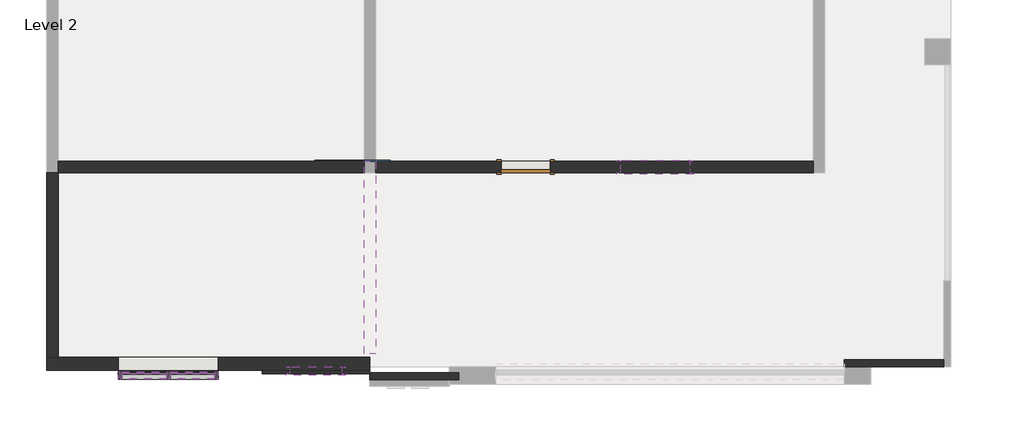
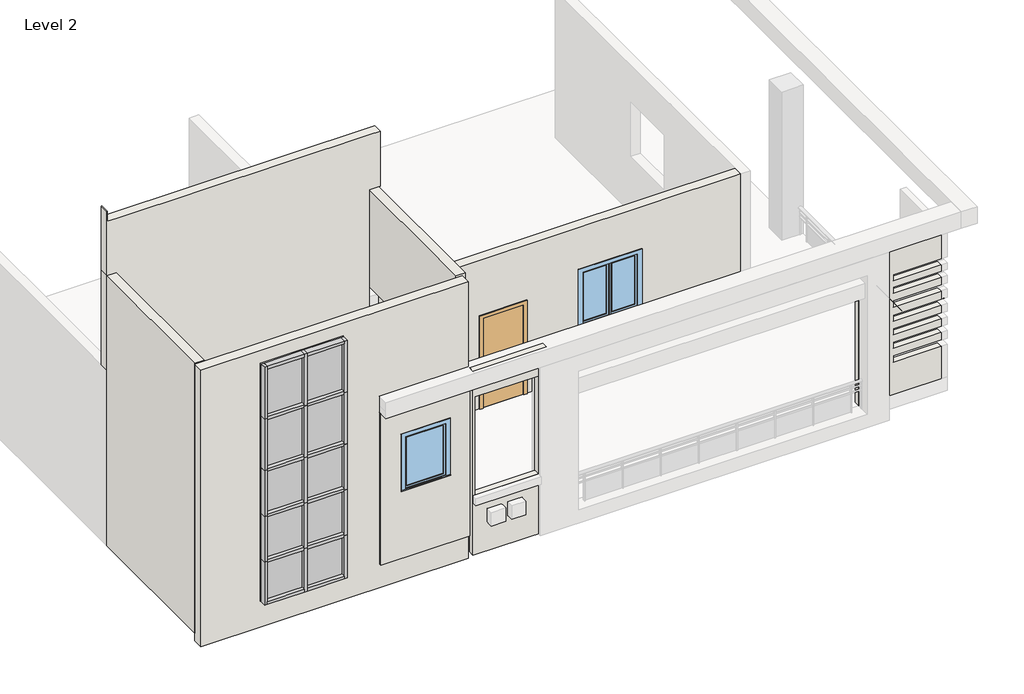
# One storey, part 1 of 2: 27 members, 10 plates, 8 walls, 3 windows, 1 door.
"""IFC4 building model written with IfcOpenShell, lengths in millimetres."""

from ifc_helpers import new_model, si_unit, frame, origin, place, context, project, spatial, polyline, outline, extrude, faceted_brep, transform, mapped, element, save
from components import door_10fd3a06, member_c3a135b3, member_e9460d8e, member_90be0342, member_476d3acb, member_bc9734be, member_9ad71e68, member_76e31e9c, member_801d2a92, system_panel_glazed_0c055d28, system_panel_glazed_6fa9ab24, system_panel_glazed_6a49b045, system_panel_glazed_66480490, window_0862ab64, window_2df9a94c

model = new_model("IFC4")

# Units and contexts
model_context = context("Model", 3, world=origin())
ifc_project = project(units=[si_unit("LENGTHUNIT", "METRE", prefix="MILLI")], contexts=[model_context])

# Site, building, storey
site = spatial("IfcSite", under=ifc_project)
building = spatial("IfcBuilding", under=site)
storey = spatial("IfcBuildingStorey", under=building, Name="Level 2", Elevation=3657.6)

# Door
placement = place(None, origin())
door_shape = door_10fd3a06(model_context)
element("IfcDoor", 1, ObjectType="Door-Single-Panel : 34\" x 80\"", at=placement, inside=storey, context=model_context, shape_type="MappedRepresentation", body=[
    mapped(door_shape, transform((-5364.932483, -170.4259649, 3962.4), x_axis=(-1.0, 0.0, 0.0), y_axis=(0.0, -1.0, 0.0), z_axis=(0.0, 0.0, 1.0))),
])

# Members
member_shape = member_c3a135b3(model_context)
element("IfcMember", 2, ObjectType="Rectangular Mullion : 2.5\" x 5\" rectangular", at=placement, inside=storey, context=model_context, shape_type="MappedRepresentation", body=[
    mapped(member_shape, transform((-11644.6696597, -3853.4259649, 4077.497679), x_axis=(0.0, 0.0, -1.0), y_axis=(0.0, -1.0, 0.0), z_axis=(-1.0, 0.0, 0.0))),
])
element("IfcMember", 3, ObjectType="Rectangular Mullion : 2.5\" x 5\" rectangular", at=placement, inside=storey, context=model_context, shape_type="MappedRepresentation", body=[
    mapped(member_shape, transform((-12496.8288845, -3853.4259649, 4077.497679), x_axis=(0.0, 0.0, -1.0), y_axis=(0.0, -1.0, 0.0), z_axis=(-1.0, 0.0, 0.0))),
])
element("IfcMember", 4, ObjectType="Rectangular Mullion : 2.5\" x 5\" rectangular", at=placement, inside=storey, context=model_context, shape_type="MappedRepresentation", body=[
    mapped(member_shape, transform((-11708.1696597, -3853.4259649, 9448.8), x_axis=(0.0, 0.0, 1.0), y_axis=(0.0, -1.0, 0.0), z_axis=(1.0, 0.0, 0.0))),
])
element("IfcMember", 5, ObjectType="Rectangular Mullion : 2.5\" x 5\" rectangular", at=placement, inside=storey, context=model_context, shape_type="MappedRepresentation", body=[
    mapped(member_shape, transform((-10856.0104349, -3853.4259649, 9448.8), x_axis=(0.0, 0.0, 1.0), y_axis=(0.0, -1.0, 0.0), z_axis=(1.0, 0.0, 0.0))),
])
member_2_shape = member_e9460d8e(model_context)
element("IfcMember", 6, ObjectType="Rectangular Mullion : 2.5\" x 5\" rectangular", at=placement, inside=storey, context=model_context, shape_type="MappedRepresentation", body=[
    mapped(member_2_shape, transform((-11676.4196597, -3853.4259649, 8280.4), x_axis=(1.0, 0.0, 0.0), y_axis=(0.0, -1.0, 0.0), z_axis=(0.0, 0.0, -1.0))),
])
member_3_shape = member_90be0342(model_context)
element("IfcMember", 7, ObjectType="Rectangular Mullion : 2.5\" x 5\" rectangular", at=placement, inside=storey, context=model_context, shape_type="MappedRepresentation", body=[
    mapped(member_3_shape, transform((-10856.0104349, -3853.4259649, 8280.4), x_axis=(0.0, 0.0, 1.0), y_axis=(0.0, -1.0, 0.0), z_axis=(1.0, 0.0, 0.0))),
])
element("IfcMember", 8, ObjectType="Rectangular Mullion : 2.5\" x 5\" rectangular", at=placement, inside=storey, context=model_context, shape_type="MappedRepresentation", body=[
    mapped(member_3_shape, transform((-11708.1696597, -3853.4259649, 8280.4), x_axis=(0.0, 0.0, 1.0), y_axis=(0.0, -1.0, 0.0), z_axis=(1.0, 0.0, 0.0))),
])
element("IfcMember", 9, ObjectType="Rectangular Mullion : 2.5\" x 5\" rectangular", at=placement, inside=storey, context=model_context, shape_type="MappedRepresentation", body=[
    mapped(member_3_shape, transform((-10856.0104349, -3853.4259649, 7112.0), x_axis=(0.0, 0.0, 1.0), y_axis=(0.0, -1.0, 0.0), z_axis=(1.0, 0.0, 0.0))),
])
element("IfcMember", 10, ObjectType="Rectangular Mullion : 2.5\" x 5\" rectangular", at=placement, inside=storey, context=model_context, shape_type="MappedRepresentation", body=[
    mapped(member_3_shape, transform((-11708.1696597, -3853.4259649, 7112.0), x_axis=(0.0, 0.0, 1.0), y_axis=(0.0, -1.0, 0.0), z_axis=(1.0, 0.0, 0.0))),
])
element("IfcMember", 11, ObjectType="Rectangular Mullion : 2.5\" x 5\" rectangular", at=placement, inside=storey, context=model_context, shape_type="MappedRepresentation", body=[
    mapped(member_3_shape, transform((-10856.0104349, -3853.4259649, 6083.565893), x_axis=(0.0, 0.0, 1.0), y_axis=(0.0, -1.0, 0.0), z_axis=(1.0, 0.0, 0.0))),
])
element("IfcMember", 12, ObjectType="Rectangular Mullion : 2.5\" x 5\" rectangular", at=placement, inside=storey, context=model_context, shape_type="MappedRepresentation", body=[
    mapped(member_3_shape, transform((-11708.1696597, -3853.4259649, 6083.565893), x_axis=(0.0, 0.0, 1.0), y_axis=(0.0, -1.0, 0.0), z_axis=(1.0, 0.0, 0.0))),
])
element("IfcMember", 13, ObjectType="Rectangular Mullion : 2.5\" x 5\" rectangular", at=placement, inside=storey, context=model_context, shape_type="MappedRepresentation", body=[
    mapped(member_3_shape, transform((-10856.0104349, -3853.4259649, 5055.131786), x_axis=(0.0, 0.0, 1.0), y_axis=(0.0, -1.0, 0.0), z_axis=(1.0, 0.0, 0.0))),
])
element("IfcMember", 14, ObjectType="Rectangular Mullion : 2.5\" x 5\" rectangular", at=placement, inside=storey, context=model_context, shape_type="MappedRepresentation", body=[
    mapped(member_3_shape, transform((-11708.1696597, -3853.4259649, 5055.131786), x_axis=(0.0, 0.0, 1.0), y_axis=(0.0, -1.0, 0.0), z_axis=(1.0, 0.0, 0.0))),
])
member_4_shape = member_476d3acb(model_context)
element("IfcMember", 15, ObjectType="Rectangular Mullion : 2.5\" x 5\" rectangular", at=placement, inside=storey, context=model_context, shape_type="MappedRepresentation", body=[
    mapped(member_4_shape, transform((-12560.3288845, -3853.4259649, 9448.8), x_axis=(-1.0, 0.0, 0.0), y_axis=(0.0, -1.0, 0.0), z_axis=(0.0, 0.0, 1.0))),
])
element("IfcMember", 16, ObjectType="Rectangular Mullion : 2.5\" x 5\" rectangular", at=placement, inside=storey, context=model_context, shape_type="MappedRepresentation", body=[
    mapped(member_4_shape, transform((-10792.5104349, -3853.4259649, 8280.4), x_axis=(1.0, 0.0, 0.0), y_axis=(0.0, -1.0, 0.0), z_axis=(0.0, 0.0, -1.0))),
])
element("IfcMember", 17, ObjectType="Rectangular Mullion : 2.5\" x 5\" rectangular", at=placement, inside=storey, context=model_context, shape_type="MappedRepresentation", body=[
    mapped(member_2_shape, transform((-11676.4196597, -3853.4259649, 7112.0), x_axis=(1.0, 0.0, 0.0), y_axis=(0.0, -1.0, 0.0), z_axis=(0.0, 0.0, -1.0))),
])
element("IfcMember", 18, ObjectType="Rectangular Mullion : 2.5\" x 5\" rectangular", at=placement, inside=storey, context=model_context, shape_type="MappedRepresentation", body=[
    mapped(member_4_shape, transform((-12560.3288845, -3853.4259649, 8280.4), x_axis=(-1.0, 0.0, 0.0), y_axis=(0.0, -1.0, 0.0), z_axis=(0.0, 0.0, 1.0))),
])
element("IfcMember", 19, ObjectType="Rectangular Mullion : 2.5\" x 5\" rectangular", at=placement, inside=storey, context=model_context, shape_type="MappedRepresentation", body=[
    mapped(member_4_shape, transform((-10792.5104349, -3853.4259649, 7112.0), x_axis=(1.0, 0.0, 0.0), y_axis=(0.0, -1.0, 0.0), z_axis=(0.0, 0.0, -1.0))),
])
member_5_shape = member_bc9734be(model_context)
element("IfcMember", 20, ObjectType="Rectangular Mullion : 2.5\" x 5\" rectangular", at=placement, inside=storey, context=model_context, shape_type="MappedRepresentation", body=[
    mapped(member_5_shape, transform((-11676.4196597, -3853.4259649, 6083.565893), x_axis=(1.0, 0.0, 0.0), y_axis=(0.0, -1.0, 0.0), z_axis=(0.0, 0.0, -1.0))),
])
element("IfcMember", 21, ObjectType="Rectangular Mullion : 2.5\" x 5\" rectangular", at=placement, inside=storey, context=model_context, shape_type="MappedRepresentation", body=[
    mapped(member_5_shape, transform((-11676.4196597, -3853.4259649, 5055.131786), x_axis=(1.0, 0.0, 0.0), y_axis=(0.0, -1.0, 0.0), z_axis=(0.0, 0.0, -1.0))),
])
member_6_shape = member_9ad71e68(model_context)
element("IfcMember", 22, ObjectType="Rectangular Mullion : 2.5\" x 5\" rectangular", at=placement, inside=storey, context=model_context, shape_type="MappedRepresentation", body=[
    mapped(member_6_shape, transform((-12560.3288845, -3853.4259649, 7112.0), x_axis=(-1.0, 0.0, 0.0), y_axis=(0.0, -1.0, 0.0), z_axis=(0.0, 0.0, 1.0))),
])
element("IfcMember", 23, ObjectType="Rectangular Mullion : 2.5\" x 5\" rectangular", at=placement, inside=storey, context=model_context, shape_type="MappedRepresentation", body=[
    mapped(member_6_shape, transform((-12560.3288845, -3853.4259649, 6083.565893), x_axis=(-1.0, 0.0, 0.0), y_axis=(0.0, -1.0, 0.0), z_axis=(0.0, 0.0, 1.0))),
])
element("IfcMember", 24, ObjectType="Rectangular Mullion : 2.5\" x 5\" rectangular", at=placement, inside=storey, context=model_context, shape_type="MappedRepresentation", body=[
    mapped(member_6_shape, transform((-10792.5104349, -3853.4259649, 6083.565893), x_axis=(1.0, 0.0, 0.0), y_axis=(0.0, -1.0, 0.0), z_axis=(0.0, 0.0, -1.0))),
])
element("IfcMember", 25, ObjectType="Rectangular Mullion : 2.5\" x 5\" rectangular", at=placement, inside=storey, context=model_context, shape_type="MappedRepresentation", body=[
    mapped(member_6_shape, transform((-10792.5104349, -3853.4259649, 5055.131786), x_axis=(1.0, 0.0, 0.0), y_axis=(0.0, -1.0, 0.0), z_axis=(0.0, 0.0, -1.0))),
])
member_7_shape = member_76e31e9c(model_context)
element("IfcMember", 26, ObjectType="Rectangular Mullion : 2.5\" x 5\" rectangular", at=placement, inside=storey, context=model_context, shape_type="MappedRepresentation", body=[
    mapped(member_7_shape, transform((-11676.4196597, -3853.4259649, 4077.497679), x_axis=(1.0, 0.0, 0.0), y_axis=(0.0, -1.0, 0.0), z_axis=(0.0, 0.0, -1.0))),
])
member_8_shape = member_801d2a92(model_context)
element("IfcMember", 27, ObjectType="Rectangular Mullion : 2.5\" x 5\" rectangular", at=placement, inside=storey, context=model_context, shape_type="MappedRepresentation", body=[
    mapped(member_8_shape, transform((-10792.5104349, -3853.4259649, 4077.497679), x_axis=(1.0, 0.0, 0.0), y_axis=(0.0, -1.0, 0.0), z_axis=(0.0, 0.0, -1.0))),
])
element("IfcMember", 28, ObjectType="Rectangular Mullion : 2.5\" x 5\" rectangular", at=placement, inside=storey, context=model_context, shape_type="MappedRepresentation", body=[
    mapped(member_8_shape, transform((-12560.3288845, -3853.4259649, 5055.131786), x_axis=(-1.0, 0.0, 0.0), y_axis=(0.0, -1.0, 0.0), z_axis=(0.0, 0.0, 1.0))),
])

# Plates
system_panel_glazed_shape = system_panel_glazed_0c055d28(model_context)
element("IfcPlate", 29, ObjectType="System Panel : Glazed", at=placement, inside=storey, context=model_context, shape_type="MappedRepresentation", body=[
    mapped(system_panel_glazed_shape, transform((-12102.4992721, -3853.4259649, 8312.15), x_axis=(1.0, 0.0, 0.0), y_axis=(0.0, 1.0, 0.0), z_axis=(0.0, 0.0, 1.0))),
])
element("IfcPlate", 30, ObjectType="System Panel : Glazed", at=placement, inside=storey, context=model_context, shape_type="MappedRepresentation", body=[
    mapped(system_panel_glazed_shape, transform((-11250.3400473, -3853.4259649, 8312.15), x_axis=(1.0, 0.0, 0.0), y_axis=(0.0, 1.0, 0.0), z_axis=(0.0, 0.0, 1.0))),
])
system_panel_glazed_2_shape = system_panel_glazed_6fa9ab24(model_context)
element("IfcPlate", 31, ObjectType="System Panel : Glazed", at=placement, inside=storey, context=model_context, shape_type="MappedRepresentation", body=[
    mapped(system_panel_glazed_2_shape, transform((-12102.4992721, -3853.4259649, 7143.75), x_axis=(1.0, 0.0, 0.0), y_axis=(0.0, 1.0, 0.0), z_axis=(0.0, 0.0, 1.0))),
])
element("IfcPlate", 32, ObjectType="System Panel : Glazed", at=placement, inside=storey, context=model_context, shape_type="MappedRepresentation", body=[
    mapped(system_panel_glazed_2_shape, transform((-11250.3400473, -3853.4259649, 7143.75), x_axis=(1.0, 0.0, 0.0), y_axis=(0.0, 1.0, 0.0), z_axis=(0.0, 0.0, 1.0))),
])
system_panel_glazed_3_shape = system_panel_glazed_6a49b045(model_context)
element("IfcPlate", 33, ObjectType="System Panel : Glazed", at=placement, inside=storey, context=model_context, shape_type="MappedRepresentation", body=[
    mapped(system_panel_glazed_3_shape, transform((-12102.4992721, -3853.4259649, 6115.315893), x_axis=(1.0, 0.0, 0.0), y_axis=(0.0, 1.0, 0.0), z_axis=(0.0, 0.0, 1.0))),
])
element("IfcPlate", 34, ObjectType="System Panel : Glazed", at=placement, inside=storey, context=model_context, shape_type="MappedRepresentation", body=[
    mapped(system_panel_glazed_3_shape, transform((-11250.3400473, -3853.4259649, 6115.315893), x_axis=(1.0, 0.0, 0.0), y_axis=(0.0, 1.0, 0.0), z_axis=(0.0, 0.0, 1.0))),
])
element("IfcPlate", 35, ObjectType="System Panel : Glazed", at=placement, inside=storey, context=model_context, shape_type="MappedRepresentation", body=[
    mapped(system_panel_glazed_3_shape, transform((-12102.4992721, -3853.4259649, 5086.881786), x_axis=(1.0, 0.0, 0.0), y_axis=(0.0, 1.0, 0.0), z_axis=(0.0, 0.0, 1.0))),
])
element("IfcPlate", 36, ObjectType="System Panel : Glazed", at=placement, inside=storey, context=model_context, shape_type="MappedRepresentation", body=[
    mapped(system_panel_glazed_3_shape, transform((-11250.3400473, -3853.4259649, 5086.881786), x_axis=(1.0, 0.0, 0.0), y_axis=(0.0, 1.0, 0.0), z_axis=(0.0, 0.0, 1.0))),
])
system_panel_glazed_4_shape = system_panel_glazed_66480490(model_context)
element("IfcPlate", 37, ObjectType="System Panel : Glazed", at=placement, inside=storey, context=model_context, shape_type="MappedRepresentation", body=[
    mapped(system_panel_glazed_4_shape, transform((-12102.4992721, -3853.4259649, 4140.997679), x_axis=(1.0, 0.0, 0.0), y_axis=(0.0, 1.0, 0.0), z_axis=(0.0, 0.0, 1.0))),
])
element("IfcPlate", 38, ObjectType="System Panel : Glazed", at=placement, inside=storey, context=model_context, shape_type="MappedRepresentation", body=[
    mapped(system_panel_glazed_4_shape, transform((-11250.3400473, -3853.4259649, 4140.997679), x_axis=(1.0, 0.0, 0.0), y_axis=(0.0, 1.0, 0.0), z_axis=(0.0, 0.0, 1.0))),
])

# Walls
element("IfcWall", 39, ObjectType="Generic - 4\" Brick", at=placement, inside=storey, context=model_context, shape_type="SweptSolid", body=[
    extrude(outline(polyline([(4035.6432835, -10021.1728698), (4035.6432835, -8116.1728698), (7457.6935311, -8116.1728698), (7457.6935311, -10021.1728698), (4035.6432835, -10021.1728698)]), holes=[polyline([(6780.679659, -9525.8728698), (6780.679659, -8611.4728698), (5561.479659, -8611.4728698), (5561.479659, -9525.8728698), (6780.679659, -9525.8728698)])]), frame((0.0, -3823.1106886, 0.0), z_axis=(0.0, 1.0, 0.0), x_axis=(0.0, 0.0, 1.0)), (0.0, 0.0, 1.0), 101.6),
])
element("IfcWall", 40, ObjectType="Generic - 5\"", at=placement, inside=storey, context=model_context, shape_type="SweptSolid", body=[
    extrude(outline(polyline([(7820.7521516, -8116.1728698), (3657.6, -8116.1728698), (3657.6, -6547.7228698), (7820.7521516, -6547.7228698), (7820.7521516, -8116.1728698)]), holes=[polyline([(7217.8061863, -6719.1728698), (5010.4540348, -6719.1728698), (5010.4540348, -8065.3728698), (7217.8061863, -8065.3728698), (7217.8061863, -6719.1728698)])]), frame((0.0, -3929.6259649, 0.0), z_axis=(0.0, 1.0, 0.0), x_axis=(0.0, 0.0, 1.0)), (0.0, 0.0, 1.0), 127.0),
])
element("IfcWall", 41, ObjectType="Generic - 5\"", at=placement, inside=storey, context=model_context, shape_type="Brep", body=[
    faceted_brep([(258.2694807, -3701.0259649, 3962.4), (2018.4271302, -3701.0259649, 3962.4), (2018.4271302, -3701.0259649, 4691.6184058), (994.8694807, -3701.0259649, 4691.6184058), (994.8694807, -3701.0259649, 4836.3196283), (2018.4271302, -3701.0259649, 4836.3196283), (2018.4271302, -3701.0259649, 5009.1184058), (994.8694807, -3701.0259649, 5009.1184058), (994.8694807, -3701.0259649, 5141.1196283), (2018.4271302, -3701.0259649, 5141.1196283), (2018.4271302, -3701.0259649, 5313.9184058), (994.8694807, -3701.0259649, 5313.9184058), (994.8694807, -3701.0259649, 5445.9196283), (2018.4271302, -3701.0259649, 5445.9196283), (2018.4271302, -3701.0259649, 5618.7184058), (994.8694807, -3701.0259649, 5618.7184058), (994.8694807, -3701.0259649, 5750.7196283), (2081.9271302, -3701.0259649, 5750.7196283), (2081.9271302, -3701.0259649, 5753.1), (2018.4271302, -3701.0259649, 5753.1), (2018.4271302, -3701.0259649, 5936.2184058), (994.8694807, -3701.0259649, 5936.2184058), (994.8694807, -3701.0259649, 6080.9196283), (2018.4271302, -3701.0259649, 6080.9196283), (2018.4271302, -3701.0259649, 6253.7184058), (994.8694807, -3701.0259649, 6253.7184058), (994.8694807, -3701.0259649, 6385.7196283), (2018.4271302, -3701.0259649, 6385.7196283), (2018.4271302, -3701.0259649, 6533.1184058), (994.8694807, -3701.0259649, 6533.1184058), (994.8694807, -3701.0259649, 6665.1196283), (2018.4271302, -3701.0259649, 6665.1196283), (2018.4271302, -3701.0259649, 7315.2), (258.2694807, -3701.0259649, 7315.2), (258.2694807, -3574.0259649, 3962.4), (258.2694807, -3574.0259649, 7315.2), (2018.4271302, -3574.0259649, 7315.2), (2018.4271302, -3574.0259649, 6665.1196283), (994.8694807, -3574.0259649, 6665.1196283), (994.8694807, -3574.0259649, 6533.1184058), (2018.4271302, -3574.0259649, 6533.1184058), (2018.4271302, -3574.0259649, 6385.7196283), (994.8694807, -3574.0259649, 6385.7196283), (994.8694807, -3574.0259649, 6253.7184058), (2018.4271302, -3574.0259649, 6253.7184058), (2018.4271302, -3574.0259649, 6080.9196283), (994.8694807, -3574.0259649, 6080.9196283), (994.8694807, -3574.0259649, 5936.2184058), (2018.4271302, -3574.0259649, 5936.2184058), (2018.4271302, -3574.0259649, 5753.1), (2081.9271302, -3574.0259649, 5753.1), (2081.9271302, -3574.0259649, 5750.7196283), (994.8694807, -3574.0259649, 5750.7196283), (994.8694807, -3574.0259649, 5618.7184058), (2018.4271302, -3574.0259649, 5618.7184058), (2018.4271302, -3574.0259649, 5445.9196283), (994.8694807, -3574.0259649, 5445.9196283), (994.8694807, -3574.0259649, 5313.9184058), (2018.4271302, -3574.0259649, 5313.9184058), (2018.4271302, -3574.0259649, 5141.1196283), (994.8694807, -3574.0259649, 5141.1196283), (994.8694807, -3574.0259649, 5009.1184058), (2018.4271302, -3574.0259649, 5009.1184058), (2018.4271302, -3574.0259649, 4836.3196283), (994.8694807, -3574.0259649, 4836.3196283), (994.8694807, -3574.0259649, 4691.6184058), (2018.4271302, -3574.0259649, 4691.6184058), (2018.4271302, -3574.0259649, 3962.4), (2018.4271302, -3637.5259649, 6080.9196283), (2018.4271302, -3637.5259649, 6385.7196283)], [[[0, 1, 2, 3, 4, 5, 6, 7, 8, 9, 10, 11, 12, 13, 14, 15, 16, 17, 18, 19, 20, 21, 22, 23, 24, 25, 26, 27, 28, 29, 30, 31, 32, 33]], [[34, 35, 36, 37, 38, 39, 40, 41, 42, 43, 44, 45, 46, 47, 48, 49, 50, 51, 52, 53, 54, 55, 56, 57, 58, 59, 60, 61, 62, 63, 64, 65, 66, 67]], [[1, 0, 34, 67]], [[33, 32, 36, 35]], [[0, 33, 35, 34]], [[3, 2, 66, 65]], [[4, 3, 65, 64]], [[5, 4, 64, 63]], [[7, 6, 62, 61]], [[8, 7, 61, 60]], [[9, 8, 60, 59]], [[11, 10, 58, 57]], [[12, 11, 57, 56]], [[13, 12, 56, 55]], [[15, 14, 54, 53]], [[16, 15, 53, 52]], [[17, 16, 52, 51]], [[21, 20, 48, 47]], [[22, 21, 47, 46]], [[23, 22, 46, 45, 68]], [[25, 24, 44, 43]], [[26, 25, 43, 42]], [[27, 26, 42, 41, 69]], [[29, 28, 40, 39]], [[30, 29, 39, 38]], [[31, 30, 38, 37]], [[18, 17, 51, 50]], [[49, 19, 18, 50]], [[2, 1, 67, 66]], [[6, 5, 63, 62]], [[10, 9, 59, 58]], [[14, 13, 55, 54]], [[20, 19, 49, 48]], [[24, 23, 68, 45, 44]], [[28, 27, 69, 41, 40]], [[32, 31, 37, 36]]]),
])
element("IfcWall", 42, ObjectType="Generic - 8\"", at=placement, inside=storey, context=model_context, shape_type="Brep", body=[
    faceted_brep([(-8217.7728698, -68.8259649, 3657.6), (-13621.6228698, -68.8259649, 3657.6), (-13621.6228698, -68.8259649, 7620.0), (-13654.5805193, -68.8259649, 7620.0), (-13806.9805193, -68.8259649, 7620.0), (-13829.2055193, -68.8259649, 7620.0), (-13829.2055193, -68.8259649, 9753.6), (-13824.8228698, -68.8259649, 9753.6), (-13824.8228698, -68.8259649, 11202.4428486), (-13810.1555193, -68.8259649, 11202.4428486), (-13810.1555193, -68.8259649, 10972.8), (-7989.1728698, -68.8259649, 10972.8), (-7989.1728698, -68.8259649, 9731.3133194), (-8014.5728698, -68.8259649, 9731.3133194), (-8217.7728698, -68.8259649, 9731.3133194), (-8217.7728698, -68.8259649, 7542.338929), (-8217.7728698, -68.8259649, 6108.5737543), (-9030.5728698, -68.8259649, 6108.5737543), (-9030.5728698, -68.8259649, 4889.3737543), (-8217.7728698, -68.8259649, 4889.3737543), (-13621.6228698, -272.0259649, 3657.6), (-8217.7728698, -272.0259649, 3657.6), (-8217.7728698, -272.0259649, 4889.3737543), (-9030.5728698, -272.0259649, 4889.3737543), (-9030.5728698, -272.0259649, 6108.5737543), (-8217.7728698, -272.0259649, 6108.5737543), (-8217.7728698, -272.0259649, 7315.2), (-8217.7728698, -272.0259649, 9731.3133194), (-7989.1728698, -272.0259649, 9731.3133194), (-7989.1728698, -272.0259649, 10972.8), (-8217.7728698, -272.0259649, 10972.8), (-13596.2228698, -272.0259649, 10972.8), (-13810.1555193, -272.0259649, 10972.8), (-13810.1555193, -272.0259649, 11194.4859918), (-13810.1555193, -272.0259649, 11202.4428486), (-13824.8228698, -272.0259649, 11202.4428486), (-13824.8228698, -272.0259649, 11194.4859918), (-13824.8228698, -272.0259649, 9753.6), (-13829.2055193, -272.0259649, 9753.6), (-13829.2055193, -272.0259649, 7620.0), (-13824.8228698, -272.0259649, 7620.0), (-13621.6228698, -272.0259649, 7620.0)], [[[0, 1, 2, 3, 4, 5, 6, 7, 8, 9, 10, 11, 12, 13, 14, 15, 16, 17, 18, 19]], [[20, 21, 22, 23, 24, 25, 26, 27, 28, 29, 30, 31, 32, 33, 34, 35, 36, 37, 38, 39, 40, 41]], [[1, 0, 21, 20]], [[28, 27, 14, 13, 12]], [[12, 11, 29, 28]], [[5, 4, 3, 2, 41, 40, 39]], [[1, 20, 41, 2]], [[21, 0, 19, 22]], [[14, 27, 26, 25, 16, 15]], [[7, 6, 38, 37]], [[5, 39, 38, 6]], [[8, 35, 34, 9]], [[9, 34, 33, 32, 10]], [[29, 11, 10, 32, 31, 30]], [[35, 8, 7, 37, 36]], [[17, 24, 23, 18]], [[18, 23, 22, 19]], [[24, 17, 16, 25]]]),
])
element("IfcWall", 43, ObjectType="Generic - 8\"", at=placement, inside=storey, context=model_context, shape_type="Brep", body=[
    faceted_brep([(-8014.5728698, -3472.4259649, 7542.338929), (-8014.5728698, -68.8259649, 7542.338929), (-8014.5728698, -68.8259649, 9731.3133194), (-8014.5728698, -3472.4259649, 9731.3133194), (-8014.5728698, -3472.4259649, 8588.3133194), (-8217.7728698, -3472.4259649, 7542.338929), (-8217.7728698, -3472.4259649, 8588.3133194), (-8217.7728698, -3472.4259649, 9731.3133194), (-8217.7728698, -2659.6259649, 9731.3133194), (-8217.7728698, -272.0259649, 9731.3133194), (-8217.7728698, -68.8259649, 9731.3133194), (-8217.7728698, -68.8259649, 7542.338929)], [[[0, 1, 2, 3, 4]], [[5, 6, 7, 8, 9, 10, 11]], [[2, 1, 11, 10]], [[1, 0, 5, 11]], [[3, 2, 10, 9, 8, 7]], [[0, 4, 6, 5]], [[4, 3, 7, 6]]]),
])
element("IfcWall", 44, ObjectType="Generic - 8\"", at=placement, inside=storey, context=model_context, shape_type="Brep", body=[
    faceted_brep([(-13626.0055193, -3535.9259649, 3657.6), (-13626.0055193, -272.0259649, 3657.6), (-13626.0055193, -272.0259649, 9753.6), (-13626.0055193, -3535.9259649, 9753.6), (-13829.2055193, -3535.9259649, 3657.6), (-13829.2055193, -3535.9259649, 9737.2171981), (-13829.2055193, -3535.9259649, 9753.6), (-13829.2055193, -272.0259649, 9753.6), (-13829.2055193, -272.0259649, 7620.0), (-13829.2055193, -272.0259649, 3657.6), (-13824.8228698, -272.0259649, 3657.6), (-13824.8228698, -272.0259649, 9753.6)], [[[0, 1, 2, 3]], [[4, 5, 6, 7, 8, 9]], [[1, 0, 4, 9, 10]], [[3, 2, 11, 7, 6]], [[0, 3, 6, 5, 4]], [[1, 10, 9, 8, 7, 11, 2]]]),
])
element("IfcWall", 45, ObjectType="Generic - 8\"", at=placement, inside=storey, context=model_context, shape_type="SweptSolid", body=[
    extrude(outline(polyline([(3657.6, -8014.5728698), (3657.6, -284.932483), (7315.2, -284.932483), (7315.2, -8014.5728698), (6108.5737543, -8014.5728698), (6108.5737543, -7811.3728698), (4889.3737543, -7811.3728698), (4889.3737543, -8014.5728698), (3657.6, -8014.5728698)]), holes=[polyline([(6302.5026994, -3688.532483), (6302.5026994, -2469.332483), (5083.3026994, -2469.332483), (5083.3026994, -3688.532483), (6302.5026994, -3688.532483)]), polyline([(3962.4, -4933.132483), (3962.4, -5796.732483), (5994.4, -5796.732483), (5994.4, -4933.132483), (3962.4, -4933.132483)])]), frame((0.0, -272.0259649, 0.0), z_axis=(0.0, 1.0, 0.0), x_axis=(0.0, 0.0, 1.0)), (0.0, 0.0, 1.0), 203.2),
])
element("IfcWall", 46, ObjectType="Generic - 8\" - Filled", at=placement, inside=storey, context=model_context, shape_type="Brep", body=[
    faceted_brep([(-13829.2055193, -3764.5259649, 3488.8171981), (-8116.1728698, -3764.5259649, 3488.8171981), (-8116.1728698, -3764.5259649, 9737.2171981), (-13829.2055193, -3764.5259649, 9737.2171981), (-10792.5104349, -3764.5259649, 9448.8), (-10792.5104349, -3764.5259649, 4077.497679), (-12560.3288845, -3764.5259649, 4077.497679), (-12560.3288845, -3764.5259649, 9448.8), (-13829.2055193, -3535.9259649, 3488.8171981), (-13829.2055193, -3535.9259649, 3657.6), (-13829.2055193, -3535.9259649, 9737.2171981), (-8116.1728698, -3535.9259649, 9737.2171981), (-8116.1728698, -3535.9259649, 3488.8171981), (-10792.5104349, -3535.9259649, 9448.8), (-12560.3288845, -3535.9259649, 9448.8), (-12560.3288845, -3535.9259649, 4077.497679), (-10792.5104349, -3535.9259649, 4077.497679)], [[[0, 1, 2, 3], [4, 5, 6, 7]], [[8, 9, 10, 11, 12], [13, 14, 15, 16]], [[0, 3, 10, 9, 8]], [[1, 0, 8, 12]], [[3, 2, 11, 10]], [[5, 4, 13, 16]], [[6, 5, 16, 15]], [[7, 6, 15, 14]], [[4, 7, 14, 13]], [[1, 12, 11, 2]]]),
])

# Windows
window_shape = window_0862ab64(model_context)
element("IfcWindow", 47, ObjectType="Casement Dbl with Trim : 48\" x 48\"", at=placement, inside=storey, context=model_context, shape_type="MappedRepresentation", body=[
    mapped(window_shape, transform((-3078.932483, -151.3759649, 4168.9026994), x_axis=(-1.0, 0.0, 0.0), y_axis=(0.0, -1.0, 0.0), z_axis=(0.0, 0.0, 1.0))),
])
element("IfcWindow", 48, ObjectType="Casement Dbl with Trim : 48\" x 48\"", at=placement, inside=storey, context=model_context, shape_type="MappedRepresentation", body=[
    mapped(window_shape, transform((-8420.9728698, -151.3759649, 3974.9737543), x_axis=(-1.0, 0.0, 0.0), y_axis=(0.0, -1.0, 0.0), z_axis=(0.0, 0.0, 1.0))),
])
window_2_shape = window_2df9a94c(model_context)
element("IfcWindow", 49, ObjectType="Casement with Trim : 36\" x 48\"", at=placement, inside=storey, context=model_context, shape_type="MappedRepresentation", body=[
    mapped(window_2_shape, transform((-9068.6728698, -3772.3106886, 4647.079659), x_axis=(-1.0, 0.0, 0.0), y_axis=(0.0, -1.0, 0.0), z_axis=(0.0, 0.0, 1.0))),
])

save(model, "model.ifc")

# Revit data of these elements
# Type "Door-Single-Panel : 34\" x 80\""
#   Type Mark = "8"
#   Construction Type Id = "DOOR"
#   Assembly Code = "C1020300"
#   Analytic Construction = "Wooden"
#   Thickness = 0' - 2"
#   Thermal Resistance (R) = 2.5876 (h·ft²·°F)/BTU
#   Swing Angle [instance default] = 90.00°
#   Heat Transfer Coefficient (U) = 0.3865 BTU/(h·ft²·°F)
#   Height = 6' - 8"
#   Trim Projection Ext = 0' - 1"
#   Trim Projection Int = 0' - 1"
#   Trim Width = 0' - 3"
#   Width = 2' - 10"
#   Define Thermal Properties by = 1
#   Panel Material = Wood - Birch - Solid Stained Light Low Gloss
#   Trim Material = Roofing, EPDM Membrane
#   Visual Light Transmittance = 0
#   Solar Heat Gain Coefficient = 0
#   Function = (empty or 0)
#   Wall Closure = (empty or 0)
# Type "Rectangular Mullion : 2.5\" x 5\" rectangular"
#   built-in parameter 1007304 = 0.416667 (stored number, unit not read)
#   built-in parameter 1007301 = 0.104167 (stored number, unit not read)
#   built-in parameter 1007300 = 0.104167 (stored number, unit not read)
# Type "System Panel : Glazed"
#   Construction Type Id = "GSP4R"
#   Analytic Construction = "1/8 in Pilkington single glazing"
#   Visual Light Transmittance = 0.9
#   Solar Heat Gain Coefficient = 0.86
#   Heat Transfer Coefficient (U) = 1.18115 BTU/(h·ft²·°F)
# Type "Generic - 4\" Brick"
#   Assembly Code = "B2010"
#   Layers, outside or top first: 0' - 4" "Brick, Common" (function 1)
# Type "Generic - 5\""
#   Assembly Code = "B2010"
#   Layers, outside or top first: 0' - 5" no material (function 1)
# Type "Generic - 8\""
#   Assembly Code = "B2010"
#   Layers, outside or top first: 0' - 8" no material (function 1)
# Type "Generic - 8\" - Filled"
#   Assembly Code = "B2010"
#   Layers, outside or top first: 0' - 9" no material (function 1)
# Type "Casement Dbl with Trim : 48\" x 48\""
#   Type Mark = "19"
#   Construction Type Id = "GSP4R"
#   Assembly Code = "B2020100"
#   Analytic Construction = "1/8 in Pilkington single glazing"
#   Visual Light Transmittance = 0.9
#   Solar Heat Gain Coefficient = 0.78
#   Heat Transfer Coefficient (U) = 0.6496 BTU/(h·ft²·°F)
#   Height = 4' - 0"
#   Default Sill Height = 3' - 0"
#   Trim Projection - Ext. = 0' - 0 1/2"
#   Trim Projection - Int. = 0' - 0 3/4"
#   Trim Width - Exterior = 0' - 3 1/2"
#   Trim Width - Interior = 0' - 3 1/2"
#   Width = 4' - 0"
#   Window Inset = 0' - 0 3/4"
#   Define Thermal Properties by = 1
#   Glass Pane Material = Glass
#   Sash Material = Sash
#   Trim Exterior Material = Trim
#   Trim Interior Material = Trim
#   Wall Closure = (empty or 0)
# Type "Casement with Trim : 36\" x 48\""
#   Type Mark = "10"
#   Construction Type Id = "GSP4R"
#   Assembly Code = "B2020100"
#   Analytic Construction = "1/8 in Pilkington single glazing"
#   Visual Light Transmittance = 0.9
#   Solar Heat Gain Coefficient = 0.78
#   Heat Transfer Coefficient (U) = 0.6496 BTU/(h·ft²·°F)
#   Height = 4' - 0"
#   Default Sill Height = 3' - 0"
#   Trim Projection - Ext. = 0' - 0 1/2"
#   Trim Projection - Int. = 0' - 0 3/4"
#   Trim Width - Exterior = 0' - 3 1/2"
#   Trim Width - Interior = 0' - 3 1/2"
#   Width = 3' - 0"
#   Window Inset = 0' - 0 3/4"
#   Define Thermal Properties by = 1
#   Glass Pane Material = Glass
#   Sash Material = Sash
#   Trim Exterior Material = Trim
#   Trim Interior Material = Trim
#   Wall Closure = (empty or 0)
# Element 1 (IfcDoor, "Door-Single-Panel : 34\" x 80\"")
#   Swing Angle = 90.00°
#   Phase Created = New Construction
#   Materials on its faces: "Roofing, EPDM Membrane", "Wood - Birch - Solid Stained Light Low Gloss"
# Elements 2, 3, 4, 5, 6, 7, 8, 9, 10, 11, 12, 13, 14, 15, 16, 17, 18, 19, 20, 21, 22, 23, 24, 25, 26, 27, 28 (IfcMember, "Rectangular Mullion : 2.5\" x 5\" rectangular")
#   Phase Created = New Construction
#   Materials on its faces: "Roofing, EPDM Membrane"
# Elements 29, 30, 31, 32, 33, 34, 35, 36, 37, 38 (IfcPlate, "System Panel : Glazed")
#   Phase Created = New Construction
#   Materials on its faces: "Glass"
# Element 39 (IfcWall, "Generic - 4\" Brick")
#   built-in parameter 1001111 = 1' - 2.88359"
#   Top Offset = 0' - 0"
#   Base Offset = 1' - 2.88359"
#   Unconnected Height = 11' - 2.72639"
#   wall height = 11' - 2.72639"
#   Phase Created = New Construction
#   Base Constraint = Level 2
#   Materials on its faces: "Brick, Common"
# Element 40 (IfcWall, "Generic - 5\"")
#   Top Offset = 1' - 7.90363"
#   Base Offset = 0' - 0"
#   wall height = 13' - 7.90363"
#   Phase Created = New Construction
#   Base Constraint = Level 2
#   Top Constraint = Level 3
#   Materials on its faces: "Default Wall"
# Element 41 (IfcWall, "Generic - 5\"")
#   built-in parameter 1001111 = 1' - 0"
#   Top Offset = 0' - 0"
#   Base Offset = 1' - 0"
#   wall height = 11' - 0"
#   Phase Created = New Construction
#   Base Constraint = Level 2
#   Top Constraint = Level 3
#   Materials on its faces: "Default Wall"
# Element 42 (IfcWall, "Generic - 8\"")
#   Top Offset = 0' - 0"
#   Base Offset = 0' - 0"
#   Unconnected Height = 24' - 9.04106"
#   wall height = 24' - 9.04106"
#   Phase Created = New Construction
#   Base Constraint = Level 2
#   Materials on its faces: "Default Wall"
# Element 43 (IfcWall, "Generic - 8\"")
#   built-in parameter 1001111 = 12' - 8.94248"
#   Top Offset = 0' - 0"
#   Base Offset = 12' - 8.94248"
#   Unconnected Height = 7' - 2.18009"
#   wall height = 7' - 2.18009"
#   Phase Created = New Construction
#   Base Constraint = Level 2
#   Materials on its faces: "Default Wall"
# Element 44 (IfcWall, "Generic - 8\"")
#   Top Offset = 0' - 0"
#   Base Offset = 0' - 0"
#   Unconnected Height = 20' - 0"
#   wall height = 20' - 0"
#   Phase Created = New Construction
#   Base Constraint = Level 2
#   Materials on its faces: "Default Wall"
# Element 45 (IfcWall, "Generic - 8\"")
#   Top Offset = 0' - 0"
#   Base Offset = 0' - 0"
#   Unconnected Height = 12' - 0"
#   wall height = 12' - 0"
#   Phase Created = New Construction
#   Base Constraint = Level 2
#   Materials on its faces: "Default Wall"
# Element 46 (IfcWall, "Generic - 8\" - Filled")
#   built-in parameter 1001111 = -0' - 6.64499"
#   Top Offset = 0' - 0"
#   Base Offset = -0' - 6.64499"
#   Unconnected Height = 20' - 6"
#   wall height = 20' - 6"
#   Phase Created = New Construction
#   Base Constraint = Level 2
#   Materials on its faces: "Default Wall"
# Element 47 (IfcWindow, "Casement Dbl with Trim : 48\" x 48\"")
#   Mark = "3"
#   Phase Created = New Construction
#   Materials on its faces: "Sash", "Trim", "Glass"
# Element 48 (IfcWindow, "Casement Dbl with Trim : 48\" x 48\"")
#   Mark = "4"
#   Phase Created = New Construction
#   Materials on its faces: "Sash", "Trim", "Glass"
# Element 49 (IfcWindow, "Casement with Trim : 36\" x 48\"")
#   Mark = "2"
#   Phase Created = New Construction
#   Materials on its faces: "Sash", "Trim", "Glass"
# Materials
#   "Wood - Birch - Solid Stained Light Low Gloss": class "Wood", colour RGB 210 159 95, transparency 0, Cost = 0
#   "Roofing, EPDM Membrane": class "Generic", colour RGB 127 127 127, transparency 0, Description = "EPDM roof membrane", Cost = 0
#   "Brick, Common": class "Masonry", colour RGB 0 0 0, transparency 0, Description = "Common brick", Cost = 0
#   "Glass": class "Glass", colour RGB 0 128 192, transparency 0.75, Description = "Soda Lime Glass", Cost = 0
#   "Sash": class "Wood", colour RGB 224 178 126, transparency 0
#   "Trim": class "Wood", colour RGB 224 178 126, transparency 0
#   "Default Wall": colour RGB 128 128 128, transparency 0
